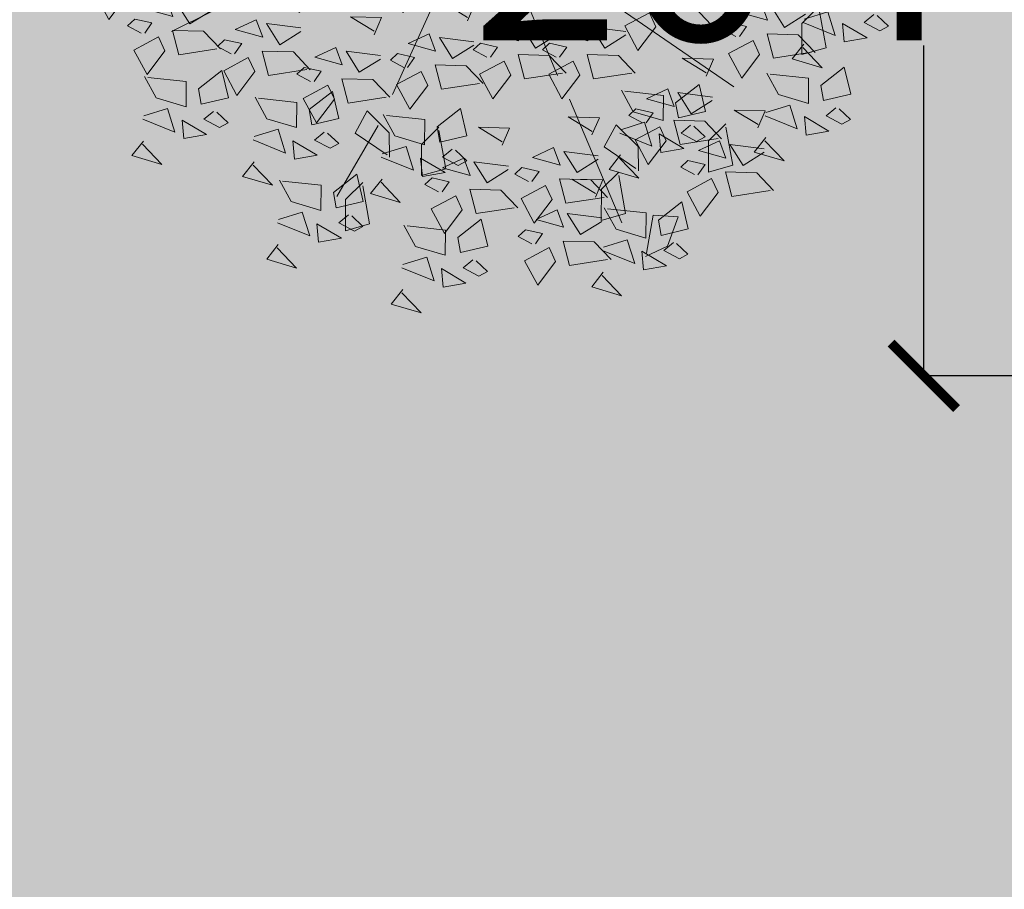
# Model space of a CAD drawing. Units: inches. Extents: x 1704 to 6393, y -157 to 1172.
# Tile 75 of 122: x 1987 to 2017, y 983 to 1009. Entities that reach past the tile are written whole.
import ezdxf

# ---------------------------------------------------------------- set-up
doc = ezdxf.new("R2010")
doc.units = ezdxf.units.IN
doc.header["$MEASUREMENT"] = 0
doc.layers.add('A-ANNO-DIMS', color=7, linetype='Continuous', lineweight=13)
doc.layers.add('L-shrub', color=74, linetype='Continuous', lineweight=18)
doc.layers.add('L-HRDS-PATT', color=9, linetype='Continuous', lineweight=13, true_color=0xc5c1ba)
doc.styles.get("Standard").update_dxf_attribs({"font": 'arial.ttf'})
doc.dimstyles.get("Standard").update_dxf_attribs({"dimtxt": 6, "dimasz": 2, "dimexe": 0.18, "dimexo": 0.0625, "dimgap": 0.09, "dimtad": 0, "dimtih": 1, "dimtoh": 1, "dimdec": 1, "dimzin": 0, "dimdsep": 46, "dimlunit": 3, "dimtxsty": 'Standard', "dimblk": 'ARCHTICK', "dimcen": 0.09, "dimadec": 0, "dimazin": 0, "dimtfac": 1, "dimtdec": 1, "dimtofl": 0, "dimtmove": 0, "dimatfit": 3, "dimfxl": 1, "dimtolj": 1, "dimtzin": 0, "dimarcsym": 0})

# ---------------------------------------------------------------- blocks, each defined once
blk = doc.blocks.new('flower shrub 2')
at = {"layer": 'L-shrub'}
for p, q in [((-106.23, 211.82), (-92.99, 218)), ((-93.69, 216.06), (-97.6, 193.26)), ((-112.6, 194.32), (-106.23, 211.82)), ((71.95, 198.59), (86.43, 202.67)), ((86.43, 202.67), (86.36, 184.05)), ((-81.12, 192.39), (-66.64, 196.47)), ((-66.64, 196.47), (-66.71, 177.85)), ((75.99, 175.82), (71.95, 198.59)), ((-97.6, 193.26), (-112.6, 194.32)), ((-77.07, 169.62), (-81.12, 192.39)), ((86.36, 184.05), (75.99, 173.75)), ((-66.71, 177.85), (-77.08, 167.55)), ((-145.24, 163.47), (-130.76, 167.54)), ((-130.76, 167.54), (-130.83, 148.93)), ((-88.72, 152.29), (-88.87, 166.9)), ((-87.4, 165.46), (-68.26, 152.47)), ((26.45, 165.53), (40.92, 169.61)), ((30.49, 142.76), (26.45, 165.53)), ((40.92, 169.61), (40.85, 150.99)), ((-141.2, 140.7), (-145.24, 163.47)), ((60.21, 144.02), (60.06, 158.64)), ((61.53, 157.19), (80.67, 144.21)), ((-130.83, 148.93), (-141.21, 138.63)), ((-75.44, 139.25), (-88.72, 152.29)), ((-68.26, 152.47), (-75.44, 139.25)), ((40.85, 150.99), (30.48, 140.69)), ((73.5, 130.99), (60.21, 144.02)), ((80.67, 144.21), (73.5, 130.99)), ((-201.09, 93.22), (-186.61, 97.3)), ((-186.61, 97.3), (-186.68, 78.69)), ((-197.05, 70.45), (-201.09, 93.22)), ((-186.68, 78.69), (-197.06, 68.38)), ((45.73, 28.33), (45.58, 42.95)), ((47.06, 41.5), (66.19, 28.51)), ((185.43, 32.08), (198.67, 38.26)), ((197.96, 36.32), (194.06, 13.53)), ((179.06, 14.59), (185.43, 32.08)), ((59.02, 15.29), (45.73, 28.33)), ((66.19, 28.51), (59.02, 15.29)), ((194.06, 13.53), (179.06, 14.59)), ((175.38, 4.39), (189.86, 8.47)), ((189.86, 8.47), (189.78, -10.15)), ((179.42, -18.38), (175.38, 4.39)), ((189.78, -10.15), (179.41, -20.45)), ((207.07, -23.32), (206.92, -8.7)), ((208.4, -10.15), (227.53, -23.13)), ((220.36, -36.35), (207.07, -23.32)), ((227.53, -23.13), (220.36, -36.35)), ((84.36, -53.46), (98.84, -49.38)), ((98.84, -49.38), (98.77, -68)), ((88.41, -76.23), (84.36, -53.46)), ((98.77, -68), (88.4, -78.3)), ((-181.81, -93.56), (-181.96, -78.94)), ((-180.48, -80.39), (-161.34, -93.38)), ((-168.52, -106.6), (-181.81, -93.56)), ((-161.34, -93.38), (-168.52, -106.6)), ((-141.1, -107.17), (-126.62, -103.09)), ((-126.62, -103.09), (-126.7, -121.71)), ((-137.06, -129.94), (-141.1, -107.17)), ((-157.94, -124.93), (-144.7, -118.75)), ((-145.41, -120.69), (-149.31, -143.48)), ((-126.7, -121.71), (-137.07, -132.01)), ((-164.31, -142.42), (-157.94, -124.93)), ((138.15, -134.03), (152.62, -129.95)), ((142.19, -156.8), (138.15, -134.03)), ((152.62, -129.95), (152.55, -148.57)), ((-149.31, -143.48), (-164.31, -142.42)), ((-142.51, -161.74), (-142.65, -147.12)), ((-141.18, -148.57), (-122.04, -161.55)), ((152.55, -148.57), (142.18, -158.87)), ((-129.22, -174.77), (-142.51, -161.74)), ((-122.04, -161.55), (-129.22, -174.77)), ((16.1, -183.61), (30.58, -179.53)), ((30.58, -179.53), (30.51, -198.15)), ((20.14, -206.38), (16.1, -183.61)), ((30.51, -198.15), (20.14, -208.45))]:
    blk.add_line(p, q, dxfattribs=at)
for points in [[(52.15, 237.83), (59.05, 246.56), (41.2, 251.84), (52.74, 239.81)], [(-67.82, 227.5), (-60.92, 236.23), (-78.77, 241.51), (-67.23, 229.48)], [(29.03, 225.28), (27.99, 236.36), (14.33, 233.94), (29.03, 225.28)], [(-39.32, 221.12), (-28.59, 235.29), (-20.71, 220.61), (-35.41, 212.74), (-39.32, 221.12)], [(10.23, 220.07), (15.95, 224.84), (6.62, 229.76), (1.48, 226.97), (8.24, 220.66)], [(52.02, 222.79), (37.77, 218.39), (33.35, 232.62), (52.6, 224.77)], [(-90.95, 214.95), (-91.98, 226.03), (-105.64, 223.61), (-90.95, 214.95)], [(126.62, 210.97), (133.52, 219.7), (115.67, 224.99), (127.2, 212.95)], [(-109.75, 209.74), (-104.02, 214.51), (-113.35, 219.43), (-118.49, 216.64), (-111.73, 210.33)], [(-67.96, 212.46), (-82.2, 208.06), (-86.62, 222.29), (-67.37, 214.44)], [(-70.39, 219.89), (-47.54, 223.41), (-43.79, 208.84), (-62.4, 209.34), (-72.46, 219.95)], [(19.2, 206.65), (5.18, 195.71), (1.34, 211.93), (17.57, 215.74), (19.2, 206.65)], [(49.53, 199.82), (26.54, 202.32), (26.68, 217.36), (44.53, 212.08), (51.52, 199.24)], [(-70.44, 189.49), (-93.43, 191.99), (-93.29, 207.03), (-75.44, 201.75), (-68.45, 188.91)], [(-27.19, 210.46), (-31.5, 204.37), (-21.21, 202.03), (-16.97, 206.05), (-25.13, 210.4)], [(103.49, 198.43), (102.46, 209.5), (88.8, 207.08), (103.49, 198.43)], [(-100.78, 196.32), (-114.8, 185.38), (-118.63, 201.6), (-102.4, 205.41), (-100.78, 196.32)], [(-66.87, 197.06), (-54.24, 204.99), (-46.3, 192.37), (-66.93, 195)], [(-44.01, 200.58), (-40.16, 190.14), (-27.58, 196), (-44.01, 200.58)], [(16.53, 190.13), (27.26, 204.31), (35.14, 189.63), (20.44, 181.76), (16.53, 190.13)], [(84.69, 193.22), (90.42, 197.99), (81.09, 202.9), (75.95, 200.11), (82.71, 193.8)], [(126.48, 195.93), (112.24, 191.53), (107.82, 205.76), (127.07, 197.91)], [(-47.57, 123.92), (-79, 197.93)], [(-37.25, 183.93), (-26.52, 198.11), (-18.64, 183.43), (-33.34, 175.56), (-37.25, 183.93)], [(-136.54, 179.8), (-125.81, 193.98), (-117.93, 179.3), (-132.63, 171.43), (-136.54, 179.8)], [(-14.54, 188.9), (8.31, 192.42), (12.06, 177.85), (-6.55, 178.35), (-16.61, 188.96)], [(93.66, 179.79), (79.64, 168.86), (75.81, 185.07), (92.04, 188.89), (93.66, 179.79)], [(124, 172.97), (101.01, 175.46), (101.15, 190.5), (119, 185.22), (125.98, 172.38)], [(-68.32, 182.7), (-45.47, 186.22), (-41.72, 171.65), (-60.33, 172.15), (-70.39, 182.76)], [(64.56, 171.72), (71.46, 180.45), (53.61, 185.73), (65.15, 173.7)], [(-167.61, 178.57), (-144.76, 182.09), (-141.01, 167.52), (-159.62, 168.02), (-169.68, 178.63)], [(-63.13, 182.49), (-67.54, 172.28), (-48.93, 171.78), (-63.18, 180.43)], [(28.66, 179.47), (24.35, 173.38), (34.64, 171.04), (38.88, 175.06), (30.72, 179.41)], [(66.94, 139.62), (91.63, 182.23)], [(-78.16, 157.26), (-71.26, 165.99), (-89.12, 171.27), (-77.58, 159.24)], [(-25.12, 173.27), (-29.43, 167.19), (-19.14, 164.84), (-14.9, 168.86), (-23.06, 173.21)], [(-11.02, 166.07), (1.61, 174), (9.54, 161.38), (-11.08, 164.01)], [(141.1, 161.39), (148, 170.12), (130.14, 175.4), (141.68, 163.37)], [(-124.41, 169.14), (-128.72, 163.05), (-118.43, 160.71), (-114.19, 164.73), (-122.34, 169.08)], [(-64.8, 159.87), (-52.17, 167.8), (-44.24, 155.19), (-64.86, 157.81)], [(11.84, 169.59), (15.69, 159.15), (28.27, 165.01), (11.84, 169.59)], [(41.44, 159.17), (40.4, 170.25), (26.74, 167.83), (41.44, 159.17)], [(64.43, 156.68), (50.18, 152.28), (45.76, 166.51), (65.01, 158.66)], [(-165.04, 146.93), (-158.14, 155.66), (-175.99, 160.94), (-164.45, 148.91)], [(-164.09, 155.74), (-151.46, 163.67), (-143.52, 151.05), (-164.15, 153.68)], [(-141.23, 159.26), (-137.38, 148.82), (-124.8, 154.68), (-141.23, 159.26)], [(-105.51, 148.81), (-94.78, 162.99), (-86.9, 148.31), (-101.6, 140.44), (-105.51, 148.81)], [(-41.95, 163.39), (-38.09, 152.95), (-25.52, 158.81), (-41.95, 163.39)], [(22.64, 153.96), (28.36, 158.73), (19.03, 163.65), (13.89, 160.86), (20.65, 154.55)], [(117.97, 148.84), (116.93, 159.92), (103.28, 157.5), (117.97, 148.84)], [(207.29, 148.99), (214.19, 157.72), (196.34, 163.01), (207.88, 150.97)], [(-101.29, 144.71), (-102.33, 155.79), (-115.98, 153.37), (-101.29, 144.71)], [(99.17, 143.63), (104.9, 148.4), (95.57, 153.32), (90.43, 150.53), (97.19, 144.22)], [(140.96, 146.35), (126.72, 141.95), (122.3, 156.18), (141.55, 148.33)], [(-136.58, 147.58), (-113.73, 151.1), (-109.98, 136.53), (-128.59, 137.03), (-138.65, 147.64)], [(-120.09, 139.5), (-114.36, 144.27), (-123.69, 149.19), (-128.83, 146.4), (-122.07, 140.09)], [(-78.3, 142.22), (-92.54, 137.81), (-96.96, 152.05), (-77.71, 144.2)], [(-7.28, 151.5), (-11.69, 141.29), (6.92, 140.79), (-7.33, 149.44)], [(31.61, 140.54), (17.59, 129.6), (13.76, 145.82), (29.99, 149.63), (31.61, 140.54)], [(61.95, 133.71), (38.95, 136.21), (39.09, 151.25), (56.94, 145.97), (63.93, 133.13)], [(184.16, 136.45), (183.13, 147.53), (169.47, 145.1), (184.16, 136.45)], [(-188.17, 134.38), (-189.2, 145.46), (-202.86, 143.04), (-188.17, 134.38)], [(-165.18, 131.89), (-179.42, 127.48), (-183.84, 141.72), (-164.59, 133.87)], [(-61.06, 145.31), (-65.47, 135.09), (-46.86, 134.59), (-61.11, 143.24)], [(207.15, 133.95), (192.91, 129.55), (188.49, 143.78), (207.74, 135.93)], [(-206.97, 129.17), (-201.24, 133.94), (-210.57, 138.86), (-215.71, 136.07), (-208.95, 129.76)], [(-160.34, 141.17), (-164.76, 130.96), (-146.15, 130.46), (-160.4, 139.11)], [(-80.78, 119.25), (-103.77, 121.75), (-103.63, 136.79), (-85.78, 131.5), (-78.8, 118.66)], [(-93.39, 138.15), (-97.69, 132.06), (-87.4, 129.72), (-83.16, 133.74), (-91.32, 138.09)], [(108.14, 130.21), (94.12, 119.27), (90.29, 135.49), (106.52, 139.3), (108.14, 130.21)], [(93.06, 124.02), (103.79, 138.2), (111.67, 123.52), (96.98, 115.65), (93.06, 124.02)], [(138.48, 123.38), (115.49, 125.88), (115.63, 140.92), (133.48, 135.64), (140.46, 122.8)], [(165.36, 131.24), (171.09, 136.01), (161.76, 140.92), (156.62, 138.13), (163.38, 131.82)], [(-133.06, 124.75), (-120.43, 132.68), (-112.5, 120.06), (-133.12, 122.69)], [(-111.12, 126.07), (-125.14, 115.14), (-128.97, 131.36), (-112.74, 135.17), (-111.12, 126.07)], [(37.21, 115.75), (47.94, 129.93), (55.82, 115.25), (41.13, 107.38), (37.21, 115.75)], [(-198, 115.75), (-212.02, 104.81), (-215.85, 121.03), (-199.62, 124.84), (-198, 115.75)], [(-167.66, 108.92), (-190.65, 111.42), (-190.51, 126.46), (-172.66, 121.17), (-165.67, 108.33)], [(-110.21, 128.27), (-106.35, 117.83), (-93.78, 123.69), (-110.21, 128.27)], [(-53.8, 109.56), (-43.07, 123.73), (-35.19, 109.05), (-49.89, 101.18), (-53.8, 109.56)], [(-12.43, 109.56), (-1.7, 123.73), (6.18, 109.05), (-8.52, 101.18), (-12.43, 109.56)], [(61.99, 122.79), (84.85, 126.31), (88.59, 111.74), (69.98, 112.24), (59.92, 122.85)], [(174.33, 117.81), (160.31, 106.88), (156.48, 123.09), (172.71, 126.91), (174.33, 117.81)], [(204.67, 110.99), (181.68, 113.48), (181.82, 128.52), (199.67, 123.24), (206.65, 110.4)], [(6.14, 114.53), (29, 118.04), (32.74, 103.47), (14.13, 103.98), (4.07, 114.58)], [(4.49, 2.24), (58.38, 121.09)], [(140.64, 107.49), (151.37, 121.67), (159.25, 106.99), (144.55, 99.12), (140.64, 107.49)], [(-2.25, 17.94), (-145.94, 116.61)], [(105.19, 113.36), (100.89, 107.27), (111.17, 104.93), (115.42, 108.95), (107.26, 113.3)], [(-161.36, 97.16), (-150.63, 111.34), (-142.75, 96.66), (-157.45, 88.79), (-161.36, 97.16)], [(-129.32, 110.18), (-133.73, 99.97), (-115.12, 99.47), (-129.37, 108.12)], [(-84.87, 108.33), (-62.02, 111.85), (-58.27, 97.28), (-76.88, 97.78), (-86.94, 108.38)], [(-43.5, 108.33), (-20.65, 111.85), (-16.9, 97.28), (-35.51, 97.78), (-45.57, 108.38)], [(4.49, 2.24), (-40.41, 109.88)], [(65.51, 99.96), (78.14, 107.89), (86.08, 95.27), (65.46, 97.9)], [(109.57, 106.26), (132.42, 109.78), (136.17, 95.21), (117.56, 95.71), (107.5, 106.32)], [(194.42, 95.09), (205.15, 109.27), (213.03, 94.59), (198.33, 86.72), (194.42, 95.09)], [(-187.79, 91.15), (-180.89, 99.88), (-198.75, 105.16), (-187.21, 93.13)], [(49.34, 105.09), (45.04, 99.01), (55.32, 96.67), (59.57, 100.68), (51.41, 105.04)], [(88.37, 103.48), (92.23, 93.04), (104.8, 98.9), (88.37, 103.48)], [(-192.43, 95.93), (-169.58, 99.45), (-165.83, 84.88), (-184.44, 85.38), (-194.5, 95.99)], [(-99.31, 80.63), (-88.58, 94.81), (-80.7, 80.13), (-95.39, 72.26), (-99.31, 80.63)], [(-41.67, 98.9), (-45.98, 92.81), (-35.69, 90.47), (-31.45, 94.49), (-39.6, 98.84)], [(-0.3, 98.9), (-4.61, 92.81), (5.68, 90.47), (9.92, 94.49), (1.76, 98.84)], [(9.66, 91.7), (22.29, 99.62), (30.23, 87.01), (9.61, 89.63)], [(32.52, 95.21), (36.38, 84.78), (48.95, 90.64), (32.52, 95.21)], [(152.77, 96.83), (148.46, 90.75), (158.75, 88.4), (162.99, 92.42), (154.83, 96.77)], [(163.35, 93.87), (186.2, 97.38), (189.95, 82.82), (171.34, 83.32), (161.28, 93.92)], [(-210.92, 78.6), (-211.96, 89.68), (-225.62, 87.26), (-210.92, 78.6)], [(-81.35, 85.5), (-68.72, 93.43), (-60.78, 80.81), (-81.41, 83.43)], [(-58.49, 89.02), (-54.64, 78.58), (-42.06, 84.44), (-58.49, 89.02)], [(-39.98, 85.5), (-27.35, 93.43), (-19.41, 80.81), (-40.04, 83.43)], [(-17.12, 89.02), (-13.27, 78.58), (-0.69, 84.44), (-17.12, 89.02)], [(113.09, 83.43), (125.72, 91.36), (133.65, 78.75), (113.03, 81.37)], [(-229.72, 73.39), (-223.99, 78.16), (-233.32, 83.08), (-238.46, 80.29), (-231.7, 73.98)], [(-187.93, 76.11), (-202.17, 71.7), (-206.59, 85.94), (-187.34, 78.09)], [(-149.23, 86.5), (-153.54, 80.42), (-143.25, 78.07), (-139.01, 82.09), (-147.17, 86.44)], [(-130.38, 79.41), (-107.52, 82.92), (-103.78, 68.35), (-122.39, 68.86), (-132.45, 79.46)], [(69.26, 85.39), (64.84, 75.18), (83.45, 74.68), (69.2, 83.33)], [(118.58, 47.68), (190.43, 83.56)], [(135.94, 86.95), (139.8, 76.51), (152.38, 82.37), (135.94, 86.95)], [(206.55, 84.43), (202.24, 78.35), (212.53, 76.01), (216.77, 80.02), (208.61, 84.38)], [(-188.91, 73.1), (-176.28, 81.03), (-168.35, 68.42), (-188.97, 71.04)], [(-166.05, 76.62), (-162.2, 66.18), (-149.62, 72.04), (-166.05, 76.62)], [(13.41, 77.13), (8.99, 66.92), (27.6, 66.41), (13.35, 75.06)], [(166.87, 71.04), (179.5, 78.96), (187.44, 66.35), (166.81, 68.97)], [(-77.6, 70.93), (-82.02, 60.72), (-63.41, 60.22), (-77.66, 68.87)], [(-36.23, 70.93), (-40.65, 60.72), (-22.04, 60.22), (-36.29, 68.87)], [(41.35, 57.91), (52.08, 72.09), (59.96, 57.41), (45.26, 49.54), (41.35, 57.91)], [(103.41, 57.91), (114.13, 72.09), (122.01, 57.41), (107.32, 49.54), (103.41, 57.91)], [(189.73, 74.55), (193.58, 64.12), (206.16, 69.98), (189.73, 74.55)], [(217.17, 62.04), (227.9, 76.22), (235.78, 61.54), (221.08, 53.67), (217.17, 62.04)], [(-220.75, 59.96), (-234.77, 49.03), (-238.6, 65.25), (-222.37, 69.06), (-220.75, 59.96)], [(-190.41, 53.14), (-213.4, 55.64), (-213.26, 70.68), (-195.41, 65.39), (-188.43, 52.55)], [(-87.18, 69.97), (-91.48, 63.89), (-81.2, 61.54), (-76.95, 65.56), (-85.11, 69.92)], [(116.83, 68.87), (112.42, 58.65), (131.03, 58.15), (116.78, 66.8)], [(-126.86, 56.58), (-114.23, 64.5), (-106.29, 51.89), (-126.91, 54.51)], [(-104, 60.09), (-100.14, 49.66), (-87.57, 55.52), (-104, 60.09)], [(10.28, 56.68), (33.14, 60.2), (36.88, 45.63), (18.27, 46.13), (8.21, 56.74)], [(72.33, 56.68), (95.19, 60.2), (98.94, 45.63), (80.33, 46.13), (70.27, 56.74)], [(186.1, 60.81), (208.96, 64.33), (212.7, 49.76), (194.09, 50.26), (184.03, 60.87)], [(-185.17, 58.54), (-189.58, 48.32), (-170.97, 47.82), (-185.22, 56.47)], [(170.61, 56.47), (166.2, 46.26), (184.81, 45.75), (170.56, 54.41)], [(-221.35, 33.12), (-210.62, 47.29), (-202.74, 32.61), (-217.44, 24.74), (-221.35, 33.12)], [(-127.81, 33.3), (-120.91, 42.03), (-138.76, 47.31), (-127.22, 35.28)], [(15.72, 2.24), (121.24, 49.33)], [(53.48, 47.25), (49.18, 41.16), (59.46, 38.82), (63.71, 42.84), (55.55, 47.19)], [(115.53, 47.25), (111.23, 41.16), (121.51, 38.82), (125.76, 42.84), (117.6, 47.19)], [(229.3, 51.38), (225, 45.3), (235.28, 42.95), (239.53, 46.97), (231.37, 51.32)], [(256.93, 35.37), (263.83, 44.1), (245.98, 49.38), (257.52, 37.35)], [(-123.11, 42.01), (-127.53, 31.79), (-108.92, 31.29), (-123.17, 39.94)], [(13.8, 33.85), (26.43, 41.78), (34.37, 29.16), (13.74, 31.79)], [(75.86, 33.85), (88.48, 41.78), (96.42, 29.16), (75.8, 31.79)], [(189.62, 37.98), (202.25, 45.91), (210.19, 33.29), (189.57, 35.92)], [(212.48, 41.5), (216.34, 31.06), (228.91, 36.92), (212.48, 41.5)], [(-252.42, 31.89), (-229.56, 35.41), (-225.82, 20.84), (-244.43, 21.34), (-254.49, 31.94)], [(36.66, 37.37), (40.51, 26.93), (53.09, 32.79), (36.66, 37.37)], [(98.71, 37.37), (102.57, 26.93), (115.14, 32.79), (98.71, 37.37)], [(-150.93, 20.75), (-151.97, 31.83), (-165.63, 29.41), (-150.93, 20.75)], [(-55.87, 20.72), (-45.14, 34.9), (-37.26, 20.22), (-51.96, 12.35), (-55.87, 20.72)], [(130.3, 16.59), (141.02, 30.77), (148.91, 16.09), (134.21, 8.22), (130.3, 16.59)], [(233.81, 22.82), (232.77, 33.9), (219.11, 31.48), (233.81, 22.82)], [(256.8, 20.33), (242.55, 15.92), (238.13, 30.16), (257.38, 22.31)], [(-169.73, 15.55), (-164.01, 20.31), (-173.34, 25.23), (-178.48, 22.44), (-171.72, 16.13)], [(-127.94, 18.26), (-142.19, 13.86), (-146.61, 28.09), (-127.36, 20.24)], [(215.01, 17.61), (220.73, 22.38), (211.4, 27.3), (206.26, 24.51), (213.02, 18.2)], [(-209.22, 22.46), (-213.52, 16.37), (-203.24, 14.03), (-198.99, 18.05), (-207.15, 22.4)], [(-86.94, 19.49), (-64.08, 23.01), (-60.34, 8.44), (-78.95, 8.94), (-89.01, 19.55)], [(17.55, 19.28), (13.13, 9.07), (31.74, 8.57), (17.49, 17.22)], [(20.21, 2.24), (132.47, 20.18)], [(79.6, 19.28), (75.19, 9.07), (93.8, 8.57), (79.54, 17.22)], [(99.22, 15.36), (122.08, 18.88), (125.83, 4.31), (107.22, 4.81), (97.16, 15.42)], [(193.37, 23.42), (188.95, 13.2), (207.56, 12.7), (193.31, 21.35)], [(-248.9, 9.06), (-236.27, 16.99), (-228.33, 4.37), (-248.95, 7)], [(-226.04, 12.58), (-222.18, 2.14), (-209.61, 8), (-226.04, 12.58)], [(-130.42, -4.7), (-153.42, -2.21), (-153.28, 12.83), (-135.43, 7.55), (-128.44, -5.29)], [(-96.78, 2.31), (-89.88, 11.04), (-107.73, 16.33), (-96.19, 4.29)], [(91.45, 0.25), (98.35, 8.98), (80.5, 14.26), (92.04, 2.23)], [(223.98, 4.18), (209.96, -6.75), (206.13, 9.47), (222.35, 13.28), (223.98, 4.18)], [(254.32, -2.64), (231.32, -0.14), (231.46, 14.9), (249.31, 9.61), (256.3, -3.23)], [(-160.76, 2.12), (-174.78, -8.81), (-178.61, 7.4), (-162.38, 11.22), (-160.76, 2.12)], [(-43.74, 10.06), (-48.04, 3.98), (-37.76, 1.63), (-33.51, 5.65), (-41.67, 10)], [(142.42, 5.93), (138.12, -0.16), (148.4, -2.5), (152.65, 1.52), (144.49, 5.87)], [(161.32, -4.07), (172.05, 10.11), (179.93, -4.57), (165.24, -12.44), (161.32, -4.07)], [(0, 0), (-177.37, -53.82)], [(-119.91, -10.23), (-120.94, 0.84), (-134.6, -1.58), (-119.91, -10.23)], [(-83.42, -3.34), (-70.79, 4.59), (-62.85, -8.02), (-83.47, -5.4)], [(-60.56, 0.18), (-56.71, -10.26), (-44.13, -4.4), (-60.56, 0.18)], [(20.21, 0), (150.43, -130.06)], [(102.75, -7.47), (115.38, 0.46), (123.31, -12.16), (102.69, -9.53)], [(-245.15, -5.51), (-249.57, -15.72), (-230.96, -16.22), (-245.21, -7.57)], [(-173.77, -18.53), (-163.04, -4.35), (-155.16, -19.03), (-169.86, -26.9), (-173.77, -18.53)], [(4.49, -4.48), (-159.41, -94.18)], [(-138.71, -15.44), (-132.98, -10.67), (-142.31, -5.76), (-147.45, -8.55), (-140.69, -14.86)], [(-96.92, -12.73), (-111.16, -17.13), (-115.58, -2.9), (-96.33, -10.75)], [(-31.05, -18.53), (-20.32, -4.35), (-12.44, -19.03), (-27.13, -26.9), (-31.05, -18.53)], [(68.33, -12.3), (67.29, -1.22), (53.63, -3.64), (68.33, -12.3)], [(91.32, -14.79), (77.07, -19.2), (72.66, -4.96), (91.9, -12.81)], [(125.6, -3.95), (129.46, -14.39), (142.03, -8.53), (125.6, -3.95)], [(130.25, -5.3), (153.11, -1.78), (156.85, -16.35), (138.24, -15.85), (128.18, -5.24)], [(4.49, -8.97), (-40.41, -192.85)], [(49.53, -17.51), (55.25, -12.74), (45.92, -7.82), (40.78, -10.61), (47.54, -16.92)], [(-204.84, -19.76), (-181.99, -16.24), (-178.24, -30.81), (-196.85, -30.31), (-206.91, -19.7)], [(-62.12, -19.76), (-39.26, -16.24), (-35.52, -30.81), (-54.13, -30.31), (-64.19, -19.7)], [(13.47, -13.45), (127.98, -183.88)], [(173.45, -14.73), (169.15, -20.81), (179.43, -23.16), (183.68, -19.14), (175.52, -14.79)], [(211.43, -28.68), (218.32, -19.95), (200.47, -14.66), (212.01, -26.7)], [(-129.74, -28.87), (-143.76, -39.8), (-147.59, -23.59), (-131.36, -19.77), (-129.74, -28.87)], [(-99.4, -35.69), (-122.39, -33.2), (-122.25, -18.16), (-104.4, -23.44), (-97.41, -36.28)], [(-79.67, -17.9), (-84.09, -28.12), (-65.48, -28.62), (-79.73, -19.97)], [(58.5, -30.94), (44.48, -41.87), (40.65, -25.65), (56.88, -21.84), (58.5, -30.94)], [(88.84, -37.76), (65.84, -35.27), (65.98, -20.22), (83.83, -25.51), (90.82, -38.35)], [(106.49, -22.04), (102.08, -32.25), (120.69, -32.75), (106.44, -24.1)], [(133.77, -28.13), (146.4, -20.2), (154.34, -32.82), (133.72, -30.19)], [(-161.65, -29.19), (-165.95, -35.28), (-155.67, -37.62), (-151.42, -33.6), (-159.58, -29.25)], [(-18.92, -29.19), (-23.22, -35.28), (-12.94, -37.62), (-8.69, -33.6), (-16.85, -29.25)], [(156.63, -24.61), (160.49, -35.05), (173.06, -29.19), (156.63, -24.61)], [(-201.32, -42.59), (-188.69, -34.66), (-180.76, -47.28), (-201.38, -44.65)], [(-58.6, -42.59), (-45.97, -34.66), (-38.03, -47.28), (-58.65, -44.65)], [(41.35, -47.45), (52.08, -33.28), (59.96, -47.96), (45.26, -55.83), (41.35, -47.45)], [(57.96, -30.81), (163.48, -42.02)], [(188.3, -41.22), (187.26, -30.14), (173.6, -32.57), (188.3, -41.22)], [(211.29, -43.72), (197.04, -48.12), (192.63, -33.89), (211.88, -41.74)], [(-178.47, -39.07), (-174.61, -49.51), (-162.04, -43.65), (-178.47, -39.07)], [(-107.58, -51.59), (-96.85, -37.41), (-88.97, -52.09), (-103.67, -59.96), (-107.58, -51.59)], [(-35.74, -39.07), (-31.88, -49.51), (-19.31, -43.65), (-35.74, -39.07)], [(-10.36, -53.65), (0.37, -39.48), (8.25, -54.15), (-6.45, -62.02), (-10.36, -53.65)], [(116.28, -51.4), (123.17, -42.67), (105.32, -37.39), (116.86, -49.42)], [(169.5, -46.43), (175.23, -41.66), (165.89, -36.75), (160.76, -39.54), (167.52, -45.85)], [(-131.94, -57.6), (-125.04, -48.87), (-142.9, -43.59), (-131.36, -55.62)], [(10.28, -48.68), (33.14, -45.17), (36.88, -59.73), (18.27, -59.23), (8.21, -48.63)], [(137.52, -42.69), (133.1, -52.91), (151.71, -53.41), (137.46, -44.76)], [(-138.65, -52.81), (-115.8, -49.3), (-112.05, -63.87), (-130.66, -63.36), (-140.72, -52.76)], [(-41.43, -54.88), (-18.58, -51.36), (-14.83, -65.93), (-33.44, -65.43), (-43.5, -54.82)], [(93.15, -63.95), (92.11, -52.87), (78.45, -55.29), (93.15, -63.95)], [(178.47, -59.86), (164.45, -70.79), (160.62, -54.58), (176.85, -50.76), (178.47, -59.86)], [(208.81, -66.68), (185.82, -64.19), (185.95, -49.15), (203.81, -54.43), (210.79, -67.27)], [(250.73, -65.86), (257.63, -57.13), (239.78, -51.85), (251.31, -63.88)], [(-197.58, -57.16), (-201.99, -67.37), (-183.38, -67.87), (-197.63, -59.22)], [(-54.85, -57.16), (-59.27, -67.37), (-40.66, -67.87), (-54.91, -59.22)], [(53.48, -58.12), (49.18, -64.2), (59.46, -66.54), (63.71, -62.52), (55.55, -58.17)], [(116.14, -66.44), (101.89, -70.85), (97.48, -56.61), (116.73, -64.46)], [(194.42, -68.11), (205.15, -53.94), (213.03, -68.62), (198.33, -76.49), (194.42, -68.11)], [(-155.07, -70.15), (-156.11, -59.07), (-169.77, -61.49), (-155.07, -70.15)], [(-132.08, -72.64), (-146.33, -77.04), (-150.74, -62.81), (-131.49, -70.66)], [(-95.45, -62.25), (-99.76, -68.33), (-89.47, -70.68), (-85.23, -66.66), (-93.39, -62.3)], [(1.77, -64.31), (-2.54, -70.4), (7.75, -72.74), (11.99, -68.72), (3.83, -64.37)], [(13.8, -71.51), (26.43, -63.59), (34.37, -76.2), (13.74, -73.58)], [(74.35, -69.16), (80.08, -64.39), (70.74, -59.47), (65.6, -62.26), (72.37, -68.57)], [(-173.87, -75.36), (-168.14, -70.59), (-177.47, -65.67), (-182.61, -68.46), (-175.85, -74.77)], [(-135.13, -75.64), (-122.5, -67.72), (-114.56, -80.33), (-135.19, -77.71)], [(-37.91, -77.71), (-25.28, -69.78), (-17.35, -82.4), (-37.97, -79.77)], [(36.66, -67.99), (40.51, -78.43), (53.09, -72.57), (36.66, -67.99)], [(163.35, -69.34), (186.2, -65.83), (189.95, -80.39), (171.34, -79.89), (161.28, -69.29)], [(227.6, -78.41), (226.56, -67.33), (212.91, -69.75), (227.6, -78.41)], [(-112.27, -72.13), (-108.42, -82.56), (-95.84, -76.7), (-112.27, -72.13)], [(-99.31, -86.71), (-88.58, -72.53), (-80.7, -87.21), (-95.39, -95.08), (-99.31, -86.71)], [(-15.06, -74.19), (-11.2, -84.63), (1.38, -78.77), (-15.06, -74.19)], [(83.32, -82.58), (69.3, -93.52), (65.47, -77.3), (81.7, -73.49), (83.32, -82.58)], [(113.66, -89.41), (90.67, -86.91), (90.8, -71.87), (108.65, -77.16), (115.64, -90)], [(113.75, -86.71), (124.48, -72.53), (132.36, -87.21), (117.66, -95.08), (113.75, -86.71)], [(208.8, -83.62), (214.53, -78.85), (205.2, -73.93), (200.06, -76.72), (206.82, -83.03)], [(250.59, -80.9), (236.35, -85.31), (231.93, -71.07), (251.18, -78.92)], [(-164.9, -88.78), (-178.92, -99.72), (-182.75, -83.5), (-166.52, -79.68), (-164.9, -88.78)], [(-134.56, -95.61), (-157.55, -93.11), (-157.42, -78.07), (-139.56, -83.35), (-132.58, -96.19)], [(-38.86, -90.66), (-31.96, -81.92), (-49.81, -76.64), (-38.27, -88.67)], [(206.55, -78.77), (202.24, -84.86), (212.53, -87.2), (216.77, -83.18), (208.61, -78.83)], [(-173.31, -96.85), (-166.41, -88.12), (-184.27, -82.84), (-172.73, -94.87)], [(-130.38, -87.94), (-107.52, -84.42), (-103.78, -98.99), (-122.39, -98.48), (-132.45, -87.88)], [(-4.91, -140.69), (-11.65, -86.87)], [(17.55, -86.08), (13.13, -96.29), (31.74, -96.8), (17.49, -88.14)], [(64.1, -99.1), (74.83, -84.93), (82.71, -99.61), (68.02, -107.48), (64.1, -99.1)], [(82.68, -87.94), (105.53, -84.42), (109.28, -98.99), (90.67, -98.48), (80.61, -87.88)], [(166.87, -92.17), (179.5, -84.24), (187.44, -96.86), (166.81, -94.24)], [(217.77, -97.05), (203.75, -107.98), (199.92, -91.76), (216.15, -87.95), (217.77, -97.05)], [(248.11, -103.87), (225.12, -101.38), (225.26, -86.33), (243.11, -91.62), (250.09, -104.46)], [(-131.39, -90.21), (-135.8, -100.43), (-117.19, -100.93), (-131.44, -92.28)], [(-61.99, -103.2), (-63.02, -92.12), (-76.68, -94.54), (-61.99, -103.2)], [(-34.17, -92.28), (-38.58, -102.49), (-19.97, -102.99), (-34.22, -94.34)], [(189.73, -88.65), (193.58, -99.09), (206.16, -93.23), (189.73, -88.65)], [(-196.44, -109.4), (-197.48, -98.32), (-211.14, -100.74), (-196.44, -109.4)], [(-87.18, -97.37), (-91.48, -103.45), (-81.2, -105.8), (-76.95, -101.78), (-85.11, -97.42)], [(-80.79, -108.41), (-75.06, -103.64), (-84.39, -98.73), (-89.53, -101.51), (-82.77, -107.82)], [(-39, -105.7), (-53.24, -110.1), (-57.66, -95.86), (-38.41, -103.72)], [(33.03, -100.33), (55.89, -96.81), (59.63, -111.38), (41.02, -110.88), (30.96, -100.28)], [(125.88, -97.37), (121.57, -103.45), (131.86, -105.8), (136.1, -101.78), (127.94, -97.42)], [(173.73, -111.5), (184.46, -97.32), (192.34, -112), (177.65, -119.87), (173.73, -111.5)], [(-215.24, -114.61), (-209.51, -109.84), (-218.84, -104.92), (-223.98, -107.71), (-217.22, -114.02)], [(-173.45, -111.89), (-187.7, -116.3), (-192.11, -102.06), (-172.86, -109.91)], [(-126.86, -110.76), (-114.23, -102.84), (-106.29, -115.45), (-126.91, -112.83)], [(71.43, -100.32), (75.92, -136.2)], [(86.2, -110.76), (98.83, -102.84), (106.76, -115.45), (86.14, -112.83)], [(-104, -107.25), (-100.14, -117.69), (-87.57, -111.82), (-104, -107.25)], [(-41.48, -128.66), (-64.47, -126.17), (-64.33, -111.13), (-46.48, -116.41), (-39.5, -129.25)], [(76.23, -109.76), (71.93, -115.85), (82.21, -118.19), (86.46, -114.17), (78.3, -109.82)], [(109.05, -107.25), (112.91, -117.69), (125.48, -111.82), (109.05, -107.25)], [(142.66, -112.73), (165.52, -109.21), (169.26, -123.78), (150.65, -123.28), (140.59, -112.67)], [(170.61, -106.74), (166.2, -116.95), (184.81, -117.46), (170.56, -108.8)], [(-175.93, -134.86), (-198.92, -132.36), (-198.79, -117.32), (-180.93, -122.61), (-173.95, -135.45)], [(-159.29, -130.09), (-148.56, -115.91), (-140.68, -130.59), (-155.38, -138.46), (-159.29, -130.09)], [(-71.82, -121.84), (-85.84, -132.77), (-89.67, -116.56), (-73.44, -112.74), (-71.82, -121.84)], [(6.19, -128.03), (16.91, -113.85), (24.8, -128.53), (10.1, -136.4), (6.19, -128.03)], [(36.55, -123.16), (49.18, -115.23), (57.12, -127.85), (36.5, -125.22)], [(145.23, -127.84), (152.13, -119.11), (134.28, -113.83), (145.82, -125.86)], [(-206.27, -128.04), (-220.29, -138.97), (-224.12, -122.75), (-207.89, -118.94), (-206.27, -128.04)], [(59.41, -119.64), (63.27, -130.08), (75.84, -124.22), (59.41, -119.64)], [(185.86, -122.16), (181.56, -128.24), (191.84, -130.59), (196.09, -126.57), (187.93, -122.22)], [(-190.37, -131.32), (-167.51, -127.8), (-163.76, -142.37), (-182.37, -141.87), (-192.43, -131.26)], [(-123.11, -125.33), (-127.53, -135.55), (-108.92, -136.05), (-123.17, -127.4)], [(-51.73, -138.36), (-41, -124.18), (-33.12, -138.86), (-47.82, -146.73), (-51.73, -138.36)], [(-24.89, -129.25), (-2.03, -125.74), (1.72, -140.31), (-16.89, -139.8), (-26.95, -129.2)], [(89.94, -125.33), (85.53, -135.55), (104.14, -136.05), (89.89, -127.4)], [(122.11, -140.39), (121.07, -129.31), (107.41, -131.73), (122.11, -140.39)], [(146.18, -135.56), (158.81, -127.63), (166.75, -140.24), (146.13, -137.62)], [(145.1, -142.88), (130.85, -147.29), (126.44, -133.05), (145.68, -140.9)], [(169.04, -132.04), (172.9, -142.48), (185.47, -136.62), (169.04, -132.04)], [(-147.17, -140.75), (-151.47, -146.84), (-141.19, -149.18), (-136.94, -145.16), (-145.1, -140.81)], [(-82.8, -139.58), (-59.95, -136.07), (-56.2, -150.64), (-74.81, -150.13), (-84.87, -139.53)], [(-4.49, -139.03), (6.74, -226.49)], [(18.31, -138.69), (14.01, -144.77), (24.29, -147.12), (28.54, -143.1), (20.38, -138.74)], [(40.3, -137.73), (35.89, -147.94), (54.49, -148.44), (40.24, -139.79)], [(103.31, -145.6), (109.03, -140.83), (99.7, -135.91), (94.56, -138.7), (101.33, -145.01)], [(-186.84, -154.15), (-174.21, -146.22), (-166.28, -158.84), (-186.9, -156.21)], [(-21.36, -152.08), (-8.73, -144.16), (-0.8, -156.77), (-21.42, -154.15)], [(-163.99, -150.63), (-160.13, -161.07), (-147.56, -155.21), (-163.99, -150.63)], [(-100.92, -167.09), (-94.02, -158.36), (-111.87, -153.08), (-100.33, -165.11)], [(-39.6, -149.02), (-43.91, -155.1), (-33.62, -157.44), (-29.38, -153.43), (-37.54, -149.07)], [(1.49, -148.57), (5.35, -159), (17.92, -153.14), (1.49, -148.57)], [(58.36, -167.09), (65.26, -158.36), (47.41, -153.08), (58.94, -165.11)], [(112.28, -159.02), (98.26, -169.96), (94.43, -153.74), (110.66, -149.93), (112.28, -159.02)], [(142.62, -165.85), (119.63, -163.35), (119.76, -148.31), (137.61, -153.6), (144.6, -166.44)], [(149.93, -150.12), (145.52, -160.34), (164.12, -160.84), (149.87, -152.19)], [(-79.28, -162.41), (-66.65, -154.49), (-58.72, -167.1), (-79.34, -164.48)], [(-56.42, -158.9), (-52.57, -169.33), (-39.99, -163.47), (-56.42, -158.9)], [(167.99, -175.36), (174.89, -166.63), (157.04, -161.34), (168.57, -173.38)], [(-183.1, -168.72), (-187.51, -178.93), (-168.9, -179.43), (-183.15, -170.78)], [(-124.04, -179.64), (-125.08, -168.56), (-138.74, -170.98), (-124.04, -179.64)], [(-39.32, -181.74), (-28.59, -167.56), (-20.71, -182.24), (-35.41, -190.11), (-39.32, -181.74)], [(-17.62, -166.65), (-22.03, -176.87), (-3.42, -177.37), (-17.67, -168.72)], [(35.23, -179.64), (34.2, -168.56), (20.54, -170.98), (35.23, -179.64)], [(90.99, -183.81), (101.72, -169.63), (109.6, -184.31), (94.91, -192.18), (90.99, -183.81)], [(-142.84, -184.85), (-137.12, -180.08), (-146.45, -175.17), (-151.59, -177.95), (-144.83, -184.26)], [(-101.05, -182.14), (-115.3, -186.54), (-119.71, -172.3), (-100.47, -180.15)], [(16.43, -184.85), (22.16, -180.08), (12.83, -175.17), (7.69, -177.95), (14.45, -184.26)], [(58.22, -182.14), (43.98, -186.54), (39.56, -172.3), (58.81, -180.15)], [(-75.54, -176.98), (-79.95, -187.19), (-61.34, -187.7), (-75.59, -179.05)], [(-70.39, -182.97), (-47.54, -179.45), (-43.79, -194.02), (-62.4, -193.52), (-72.46, -182.91)], [(59.92, -185.03), (82.78, -181.52), (86.52, -196.09), (67.91, -195.58), (57.85, -184.98)], [(144.86, -187.9), (143.83, -176.83), (130.17, -179.25), (144.86, -187.9)], [(167.85, -190.4), (153.61, -194.8), (149.19, -180.57), (168.44, -188.42)], [(-103.53, -205.1), (-126.52, -202.61), (-126.39, -187.57), (-108.54, -192.85), (-101.55, -205.69)], [(-63.68, -200.15), (-56.78, -191.42), (-74.64, -186.14), (-63.1, -198.17)], [(55.74, -205.1), (32.75, -202.61), (32.89, -187.57), (50.74, -192.85), (57.72, -205.69)], [(126.06, -193.11), (131.79, -188.35), (122.46, -183.43), (117.32, -186.22), (124.08, -192.53)], [(-133.87, -198.28), (-147.89, -209.21), (-151.72, -192.99), (-135.49, -189.18), (-133.87, -198.28)], [(-27.19, -192.4), (-31.5, -198.49), (-21.21, -200.83), (-16.97, -196.81), (-25.13, -192.46)], [(25.4, -198.28), (11.38, -209.21), (7.55, -192.99), (23.78, -189.18), (25.4, -198.28)], [(-66.87, -205.8), (-54.24, -197.87), (-46.3, -210.49), (-66.93, -207.86)], [(63.44, -207.86), (76.07, -199.94), (84.01, -212.55), (63.39, -209.93)], [(103.12, -194.47), (98.82, -200.55), (109.1, -202.9), (113.35, -198.88), (105.19, -194.52)], [(135.03, -206.54), (121.01, -217.47), (117.18, -201.26), (133.41, -197.44), (135.03, -206.54)], [(165.37, -213.36), (142.38, -210.87), (142.52, -195.83), (160.37, -201.11), (167.35, -213.95)], [(-86.81, -212.7), (-87.85, -201.62), (-101.51, -204.04), (-86.81, -212.7)], [(-63.82, -215.19), (-78.07, -219.59), (-82.48, -205.36), (-63.23, -213.21)], [(-44.01, -202.28), (-40.16, -212.72), (-27.58, -206.86), (-44.01, -202.28)], [(86.3, -204.35), (90.16, -214.78), (102.73, -208.92), (86.3, -204.35)], [(-105.61, -217.91), (-99.88, -213.14), (-109.21, -208.22), (-114.35, -211.01), (-107.59, -217.32)], [(-96.64, -231.33), (-110.66, -242.26), (-114.49, -226.05), (-98.26, -222.23), (-96.64, -231.33)], [(-66.3, -238.16), (-89.29, -235.66), (-89.16, -220.62), (-71.3, -225.9), (-64.32, -238.74)], [(-63.13, -220.37), (-67.54, -230.58), (-48.93, -231.08), (-63.18, -222.43)], [(67.19, -222.43), (62.78, -232.65), (81.39, -233.15), (67.13, -224.5)]]:
    blk.add_lwpolyline(points, dxfattribs=at)
blk = doc.blocks.new('_ArchTick')
at = {"color": 0, "linetype": 'ByBlock', "const_width": 0.15}
blk.add_lwpolyline([(-0.5, -0.5), (0.5, 0.5)], dxfattribs=at)
blk = doc.blocks.new('*D81')
at = {"layer": 'A-ANNO-DIMS', "color": 0, "lineweight": -2, "transparency": 16777216}
for p, q in [((2018.903, 1024.938), (2014.807, 1024.938)), ((2014.987, 1024.938), (2014.987, 1014.847)), ((2014.987, 998.449), (2014.987, 1008.54)), ((2018.903, 998.449), (2014.807, 998.449))]:
    blk.add_line(p, q, dxfattribs=at)
at = {"layer": 'Defpoints', "color": 0, "lineweight": -3, "transparency": 16777216}
for p in [(2018.966, 1024.938), (2014.987, 998.449), (2018.966, 998.449)]:
    blk.add_point(p, dxfattribs=at)
at = {"layer": 'A-ANNO-DIMS', "color": 0, "lineweight": -2, "transparency": 16777216, "xscale": 2, "yscale": 2, "zscale": 2}
for p, rotation in [((2014.987, 1024.938), 90), ((2014.987, 998.449), 270)]:
    blk.add_blockref('_ArchTick', p, dxfattribs=dict(at, rotation=rotation))
at = {"layer": 'A-ANNO-DIMS', "color": 0, "transparency": 16777216, "insert": (2014.987, 1011.694), "char_height": 6, "attachment_point": 5}
blk.add_mtext('\\A1;26 TYP.', dxfattribs=at)
blk = doc.blocks.new('*D94')
at = {"layer": 'A-ANNO-DIMS', "color": 0, "lineweight": -2, "transparency": 16777216}
for p, q in [((1898.349, 895.275), (1898.349, 1105.287)), ((1898.349, 1105.107), (1979.39, 1105.107)), ((2073.349, 1105.107), (1992.307, 1105.107)), ((2073.349, 895.275), (2073.349, 1105.287))]:
    blk.add_line(p, q, dxfattribs=at)
at = {"layer": 'Defpoints', "color": 0, "lineweight": -3, "transparency": 16777216}
for p in [(2073.349, 1105.107), (1898.349, 895.213), (2073.349, 895.213)]:
    blk.add_point(p, dxfattribs=at)
at = {"layer": 'A-ANNO-DIMS', "color": 0, "lineweight": -2, "transparency": 16777216, "xscale": 2, "yscale": 2, "zscale": 2, "rotation": 180}
blk.add_blockref('_ArchTick', (1898.349, 1105.107), dxfattribs=at)
at = {"layer": 'A-ANNO-DIMS', "color": 0, "lineweight": -2, "transparency": 16777216, "xscale": 2, "yscale": 2, "zscale": 2}
blk.add_blockref('_ArchTick', (2073.349, 1105.107), dxfattribs=at)
at = {"layer": 'A-ANNO-DIMS', "color": 0, "transparency": 16777216, "insert": (1985.849, 1105.107), "char_height": 6, "attachment_point": 5}
blk.add_mtext('\\A1;175', dxfattribs=at)

msp = doc.modelspace()

# ---------------------------------------------------------------- hatches: boundary and pattern name
at = {"layer": 'L-HRDS-PATT', "transparency": 33554643}
h = msp.add_hatch(color=256, dxfattribs=at)
h.dxf.hatch_style = 1
h.paths.add_polyline_path([(2065.589, 1033.213), (1898.349, 1033.213), (1898.349, 895.213), (2065.589, 895.213)])

# ---------------------------------------------------------------- block references
at = {"layer": 'L-shrub', "xscale": 0.0510581485411622, "yscale": 0.0510581485411622, "zscale": 0.0510581485411622, "rotation": 180}
msp.add_blockref('flower shrub 2', (2001.734, 1013.227), dxfattribs=at)

# ---------------------------------------------------------------- dimensions: what is measured, and where the dimension line sits
at = {"layer": 'A-ANNO-DIMS'}
dim = msp.add_linear_dim(base=(2073.349, 1105.107), p1=(1898.349, 895.213), p2=(2073.349, 895.213), dimstyle='Standard', override={"dimdec": 0, "dimlfac": 1, "dimrnd": 0, "dimzin": 0, "dimdsep": 46, "dimlunit": 2}, dxfattribs=at)
dim.commit()
dim.dimension.update_dxf_attribs({"geometry": '*D94', "text_midpoint": (1985.849, 1105.107)})
dim = msp.add_linear_dim(base=(2014.987, 998.449), p1=(2018.966, 1024.938), p2=(2018.966, 998.449), angle=270, text='<> TYP.', dimstyle='Standard', override={"dimdec": 0, "dimlfac": 1, "dimrnd": 0, "dimzin": 0, "dimdsep": 46, "dimlunit": 2}, dxfattribs=at)
dim.commit()
dim.dimension.update_dxf_attribs({"geometry": '*D81', "text_midpoint": (2014.987, 1011.694)})

doc.saveas('drawing.dxf')
